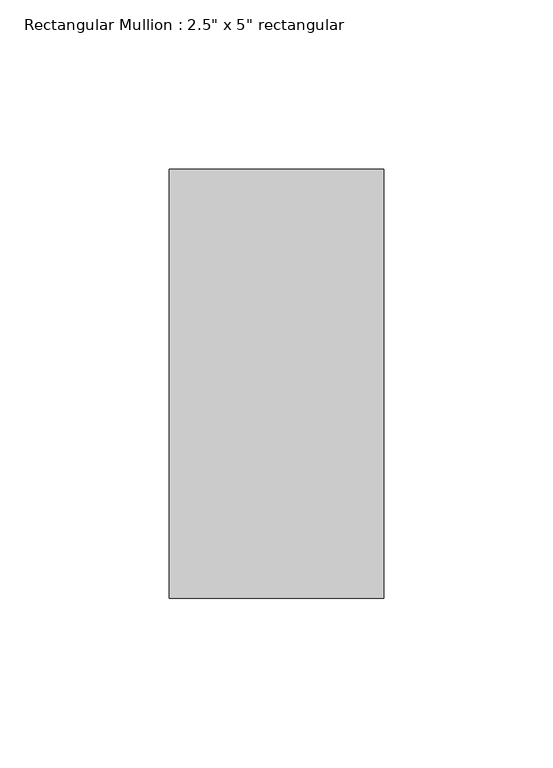
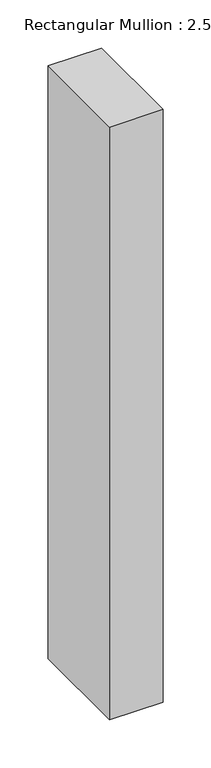
"""IFC4 building model written with IfcOpenShell, lengths in millimetres: member geometry."""

from ifc_helpers import new_model, si_unit, frame, origin, place, context, project, spatial, polyline, outline, extrude, source, transform, mapped, element, save


def member_f77fa896(model_context):
    return source(origin(), model_context, "Body", "SweptSolid", [
        extrude(outline(polyline([(0.0, 63.5), (0.0, -63.5), (-63.5, -63.5), (-63.5, 63.5), (0.0, 63.5)])), frame((0.0, 0.0, -747.8147734), z_axis=(0.0, 0.0, 1.0), x_axis=(1.0, 0.0, 0.0)), (0.0, 0.0, 1.0), 747.8147734),
    ])


if __name__ == "__main__":
    model = new_model("IFC4")
    model_context = context("Model", 3, world=origin())
    ifc_project = project(units=[si_unit("LENGTHUNIT", "METRE", prefix="MILLI")], contexts=[model_context])
    site = spatial("IfcSite", under=ifc_project)
    building = spatial("IfcBuilding", under=site)
    placement = place(None, origin())
    member_shape = member_f77fa896(model_context)
    element("IfcMember", 1, ObjectType="Rectangular Mullion : 2.5\" x 5\" rectangular", at=placement, inside=building, context=model_context, shape_type="MappedRepresentation", body=[
        mapped(member_shape, transform((0.0, 0.0, 0.0), x_axis=(1.0, 0.0, 0.0), y_axis=(0.0, 1.0, 0.0), z_axis=(0.0, 0.0, 1.0))),
    ])
    save(model, "model.ifc")

# Revit data of these elements
# Type "Rectangular Mullion : 2.5\" x 5\" rectangular"
#   built-in parameter 1007304 = 0.416667 (stored number, unit not read)
#   built-in parameter 1007301 = 0.104167 (stored number, unit not read)
#   built-in parameter 1007300 = 0.104167 (stored number, unit not read)
# Element 1 (IfcMember, "Rectangular Mullion : 2.5\" x 5\" rectangular")
#   Materials on its faces: "Aluminum"
# Materials
#   "Aluminum": class "Metal", colour RGB 247 247 247, transparency 0, Description = "Aluminum 6061", Cost = 0
